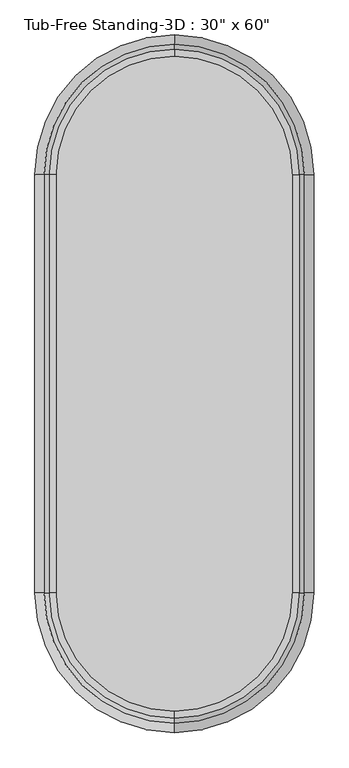
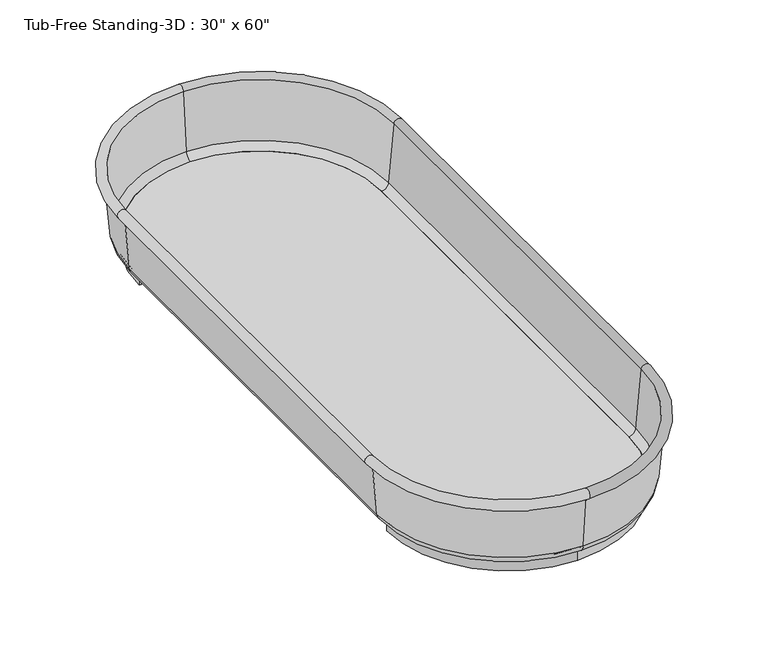
"""IFC4 building model written with IfcOpenShell, lengths in millimetres: flow terminal geometry."""

from ifc_helpers import new_model, si_unit, point, frame, frame_2d, origin, origin_with_axes, place, context, project, spatial, polyline, circle_curve, ellipse_curve, trimmed, segment, composite_curve, outline, extrude, source, transform, mapped, element, save
from ifc_brep_helpers import plane_surface, cylinder_surface, revolved_surface, advanced_brep


def flow_terminal_2cf38851(model_context):
    return source(origin(), model_context, "Body", "SolidModel", [
        advanced_brep(
        [(0.0, -1866.9, 406.4), (723.9, -1143.0, 406.4), (736.6, -1143.0, 406.4), (0.0, -1879.6, 406.4), (0.0, -1841.1045038, 111.5561295), (698.1045038, -1143.0, 111.5561295), (0.0, -1788.2824236, 63.1536107), (645.2824236, -1143.0, 63.1536107), (0.0, -1788.2824236, 78.0774627), (645.2824236, -1143.0, 78.0774627), (0.0, -1826.2374416, 112.8568289), (683.2374416, -1143.0, 112.8568289), (0.0, -1854.4561556, 435.3982063), (711.4561556, -1143.0, 435.3982063), (-723.9, -1143.0, 406.4), (-736.6, -1143.0, 406.4), (-698.1045038, -1143.0, 111.5561295), (-645.2824236, -1143.0, 63.1536107), (-645.2824236, -1143.0, 78.0774627), (-683.2374416, -1143.0, 112.8568289), (-711.4561556, -1143.0, 435.3982063), (-736.6, 1143.0, 406.4), (-723.9, 1143.0, 406.4), (-698.1045038, 1143.0, 111.5561295), (-645.2824236, 1143.0, 63.1536107), (-645.2824236, 1143.0, 78.0774627), (-683.2374416, 1143.0, 112.8568289), (-711.4561556, 1143.0, 435.3982063), (0.0, 1866.9, 406.4), (0.0, 1879.6, 406.4), (0.0, 1841.1045038, 111.5561295), (0.0, 1788.2824236, 63.1536107), (0.0, 1788.2824236, 78.0774627), (0.0, 1826.2374416, 112.8568289), (0.0, 1854.4561556, 435.3982063), (723.9, 1143.0, 406.4), (736.6, 1143.0, 406.4), (698.1045038, 1143.0, 111.5561295), (645.2824236, 1143.0, 63.1536107), (645.2824236, 1143.0, 78.0774627), (683.2374416, 1143.0, 112.8568289), (711.4561556, 1143.0, 435.3982063)],
        [
            (0, 1, circle_curve(frame((0.0, -1143.0, 406.4), z_axis=(0.0, 0.0, 1.0), x_axis=(1.0, 0.0, 0.0)), 723.9)),
            (1, 2),
            (2, 3, circle_curve(frame((0.0, -1143.0, 406.4), z_axis=(0.0, 0.0, -1.0), x_axis=(1.0, 0.0, 0.0)), 736.6)),
            (3, 0),
            (4, 5, circle_curve(frame((0.0, -1143.0, 111.5561295), z_axis=(0.0, 0.0, 1.0), x_axis=(1.0, 0.0, 0.0)), 698.1045038)),
            (5, 1),
            (0, 4),
            (6, 7, circle_curve(frame((0.0, -1143.0, 63.1536107), z_axis=(0.0, 0.0, 1.0), x_axis=(1.0, 0.0, 0.0)), 645.2824236)),
            (7, 5, circle_curve(frame((645.2824236, -1143.0, 116.1774627), z_axis=(0.0, -1.0, 0.0), x_axis=(1.0, 0.0, 0.0)), 53.023852)),
            (4, 6, circle_curve(frame((0.0, -1788.2824236, 116.1774627), z_axis=(1.0, 0.0, 0.0), x_axis=(0.0, -1.0, 0.0)), 53.023852)),
            (8, 9, circle_curve(frame((0.0, -1143.0, 78.0774627), z_axis=(0.0, 0.0, 1.0), x_axis=(1.0, 0.0, 0.0)), 645.2824236)),
            (9, 7),
            (6, 8),
            (10, 11, circle_curve(frame((0.0, -1143.0, 112.8568289), z_axis=(0.0, 0.0, 1.0), x_axis=(1.0, 0.0, 0.0)), 683.2374416)),
            (11, 9, circle_curve(frame((645.2824236, -1143.0, 116.1774627), z_axis=(0.0, 1.0, 0.0), x_axis=(1.0, 0.0, 0.0)), 38.1)),
            (8, 10, circle_curve(frame((0.0, -1788.2824236, 116.1774627), z_axis=(-1.0, 0.0, 0.0), x_axis=(0.0, -1.0, 0.0)), 38.1)),
            (12, 13, circle_curve(frame((0.0, -1143.0, 435.3982063), z_axis=(0.0, 0.0, 1.0), x_axis=(1.0, 0.0, 0.0)), 711.4561556)),
            (13, 11),
            (10, 12),
            (2, 13, circle_curve(frame((736.6, -1143.0, 431.8), z_axis=(0.0, -1.0, 0.0), x_axis=(1.0, 0.0, 0.0)), 25.4)),
            (12, 3, circle_curve(frame((0.0, -1879.6, 431.8), z_axis=(1.0, 0.0, 0.0), x_axis=(0.0, -1.0, 0.0)), 25.4)),
            (14, 0, circle_curve(frame((0.0, -1143.0, 406.4), z_axis=(0.0, 0.0, 1.0), x_axis=(0.0, -1.0, 0.0)), 723.9)),
            (3, 15, circle_curve(frame((0.0, -1143.0, 406.4), z_axis=(0.0, 0.0, -1.0), x_axis=(0.0, -1.0, 0.0)), 736.6)),
            (15, 14),
            (16, 4, circle_curve(frame((0.0, -1143.0, 111.5561295), z_axis=(0.0, 0.0, 1.0), x_axis=(0.0, -1.0, 0.0)), 698.1045038)),
            (14, 16),
            (17, 6, circle_curve(frame((0.0, -1143.0, 63.1536107), z_axis=(0.0, 0.0, 1.0), x_axis=(0.0, -1.0, 0.0)), 645.2824236)),
            (16, 17, circle_curve(frame((-645.2824236, -1143.0, 116.1774627), z_axis=(0.0, -1.0, 0.0), x_axis=(-1.0, 0.0, 0.0)), 53.023852)),
            (18, 8, circle_curve(frame((0.0, -1143.0, 78.0774627), z_axis=(0.0, 0.0, 1.0), x_axis=(0.0, -1.0, 0.0)), 645.2824236)),
            (17, 18),
            (19, 10, circle_curve(frame((0.0, -1143.0, 112.8568289), z_axis=(0.0, 0.0, 1.0), x_axis=(0.0, -1.0, 0.0)), 683.2374416)),
            (18, 19, circle_curve(frame((-645.2824236, -1143.0, 116.1774627), z_axis=(0.0, 1.0, 0.0), x_axis=(-1.0, 0.0, 0.0)), 38.1)),
            (20, 12, circle_curve(frame((0.0, -1143.0, 435.3982063), z_axis=(0.0, 0.0, 1.0), x_axis=(0.0, -1.0, 0.0)), 711.4561556)),
            (19, 20),
            (20, 15, circle_curve(frame((-736.6, -1143.0, 431.8), z_axis=(0.0, -1.0, 0.0), x_axis=(-1.0, 0.0, 0.0)), 25.4)),
            (15, 21),
            (21, 22),
            (22, 14),
            (22, 23),
            (23, 16),
            (23, 24, circle_curve(frame((-645.2824236, 1143.0, 116.1774627), z_axis=(0.0, -1.0, 0.0), x_axis=(-1.0, 0.0, 0.0)), 53.023852)),
            (24, 17),
            (24, 25),
            (25, 18),
            (25, 26, circle_curve(frame((-645.2824236, 1143.0, 116.1774627), z_axis=(0.0, 1.0, 0.0), x_axis=(-1.0, 0.0, 0.0)), 38.1)),
            (26, 19),
            (26, 27),
            (27, 20),
            (27, 21, circle_curve(frame((-736.6, 1143.0, 431.8), z_axis=(0.0, -1.0, 0.0), x_axis=(-1.0, 0.0, 0.0)), 25.4)),
            (28, 22, circle_curve(frame((0.0, 1143.0, 406.4), z_axis=(0.0, 0.0, 1.0), x_axis=(-1.0, 0.0, 0.0)), 723.9)),
            (21, 29, circle_curve(frame((0.0, 1143.0, 406.4), z_axis=(0.0, 0.0, -1.0), x_axis=(-1.0, 0.0, 0.0)), 736.6)),
            (29, 28),
            (30, 23, circle_curve(frame((0.0, 1143.0, 111.5561295), z_axis=(0.0, 0.0, 1.0), x_axis=(-1.0, 0.0, 0.0)), 698.1045038)),
            (28, 30),
            (31, 24, circle_curve(frame((0.0, 1143.0, 63.1536107), z_axis=(0.0, 0.0, 1.0), x_axis=(-1.0, 0.0, 0.0)), 645.2824236)),
            (30, 31, circle_curve(frame((0.0, 1788.2824236, 116.1774627), z_axis=(-1.0, 0.0, 0.0), x_axis=(0.0, 1.0, 0.0)), 53.023852)),
            (32, 25, circle_curve(frame((0.0, 1143.0, 78.0774627), z_axis=(0.0, 0.0, 1.0), x_axis=(-1.0, 0.0, 0.0)), 645.2824236)),
            (31, 32),
            (33, 26, circle_curve(frame((0.0, 1143.0, 112.8568289), z_axis=(0.0, 0.0, 1.0), x_axis=(-1.0, 0.0, 0.0)), 683.2374416)),
            (32, 33, circle_curve(frame((0.0, 1788.2824236, 116.1774627), z_axis=(1.0, 0.0, 0.0), x_axis=(0.0, 1.0, 0.0)), 38.1)),
            (34, 27, circle_curve(frame((0.0, 1143.0, 435.3982063), z_axis=(0.0, 0.0, 1.0), x_axis=(-1.0, 0.0, 0.0)), 711.4561556)),
            (33, 34),
            (34, 29, circle_curve(frame((0.0, 1879.6, 431.8), z_axis=(-1.0, 0.0, 0.0), x_axis=(0.0, 1.0, 0.0)), 25.4)),
            (35, 28, circle_curve(frame((0.0, 1143.0, 406.4), z_axis=(0.0, 0.0, 1.0), x_axis=(0.0, 1.0, 0.0)), 723.9)),
            (29, 36, circle_curve(frame((0.0, 1143.0, 406.4), z_axis=(0.0, 0.0, -1.0), x_axis=(0.0, 1.0, 0.0)), 736.6)),
            (36, 35),
            (37, 30, circle_curve(frame((0.0, 1143.0, 111.5561295), z_axis=(0.0, 0.0, 1.0), x_axis=(0.0, 1.0, 0.0)), 698.1045038)),
            (35, 37),
            (38, 31, circle_curve(frame((0.0, 1143.0, 63.1536107), z_axis=(0.0, 0.0, 1.0), x_axis=(0.0, 1.0, 0.0)), 645.2824236)),
            (37, 38, circle_curve(frame((645.2824236, 1143.0, 116.1774627), z_axis=(0.0, 1.0, 0.0), x_axis=(1.0, 0.0, 0.0)), 53.023852)),
            (39, 32, circle_curve(frame((0.0, 1143.0, 78.0774627), z_axis=(0.0, 0.0, 1.0), x_axis=(0.0, 1.0, 0.0)), 645.2824236)),
            (38, 39),
            (40, 33, circle_curve(frame((0.0, 1143.0, 112.8568289), z_axis=(0.0, 0.0, 1.0), x_axis=(0.0, 1.0, 0.0)), 683.2374416)),
            (39, 40, circle_curve(frame((645.2824236, 1143.0, 116.1774627), z_axis=(0.0, -1.0, 0.0), x_axis=(1.0, 0.0, 0.0)), 38.1)),
            (41, 34, circle_curve(frame((0.0, 1143.0, 435.3982063), z_axis=(0.0, 0.0, 1.0), x_axis=(0.0, 1.0, 0.0)), 711.4561556)),
            (40, 41),
            (41, 36, circle_curve(frame((736.6, 1143.0, 431.8), z_axis=(0.0, 1.0, 0.0), x_axis=(1.0, 0.0, 0.0)), 25.4)),
            (36, 2),
            (1, 35),
            (5, 37),
            (7, 38),
            (9, 39),
            (11, 40),
            (13, 41),
        ],
        [
            plane_surface(frame((0.0, -1143.0, 406.4), z_axis=(0.0, 0.0, -1.0), x_axis=(1.0, 0.0, 0.0))),
            revolved_surface(polyline([(723.9, -1143.0, 406.4), (698.1045038, -1143.0, 111.5561295)]), (0.0, -1143.0, 431.8), (0.0, 0.0, -1.0)),
            revolved_surface(trimmed(ellipse_curve(frame((645.2824236, -1143.0, 116.1774627), z_axis=(0.0, 1.0, 0.0), x_axis=(1.0, 0.0, 0.0)), 53.023852, 53.023852), [point((698.1045038, -1143.0, 111.5561295))], [point((645.2824236, -1143.0, 63.1536107))], True, "CARTESIAN"), (0.0, -1143.0, 431.8), (0.0, 0.0, -1.0)),
            revolved_surface(polyline([(645.2824236, -1143.0, 63.1536107), (645.2824236, -1143.0, 78.07746270000001)]), (0.0, -1143.0, 431.8), (0.0, 0.0, -1.0)),
            revolved_surface(trimmed(ellipse_curve(frame((645.2824236, -1143.0, 116.1774627), z_axis=(0.0, -1.0, 0.0), x_axis=(1.0, 0.0, 0.0)), 38.1, 38.1), [point((645.2824236, -1143.0, 78.0774627))], [point((683.2374416, -1143.0, 112.8568289))], True, "CARTESIAN"), (0.0, -1143.0, 431.8), (0.0, 0.0, -1.0)),
            revolved_surface(polyline([(683.2374416, -1143.0, 112.8568289), (711.4561556, -1143.0, 435.3982063)]), (0.0, -1143.0, 431.8), (0.0, 0.0, -1.0)),
            revolved_surface(trimmed(ellipse_curve(frame((736.6, -1143.0, 431.8), z_axis=(0.0, 1.0, 0.0), x_axis=(1.0, 0.0, 0.0)), 25.4, 25.4), [point((711.4561556, -1143.0, 435.3982063))], [point((736.6, -1143.0, 406.4))], True, "CARTESIAN"), (0.0, -1143.0, 431.8), (0.0, 0.0, -1.0)),
            plane_surface(frame((0.0, -1143.0, 406.4), z_axis=(0.0, 0.0, -1.0), x_axis=(0.0, -1.0, 0.0))),
            revolved_surface(polyline([(0.0, -1866.9, 406.4), (0.0, -1841.1045038, 111.5561295)]), (0.0, -1143.0, 431.8), (0.0, 0.0, -1.0)),
            revolved_surface(trimmed(ellipse_curve(frame((0.0, -1788.2824236, 116.1774627), z_axis=(1.0, 0.0, 0.0), x_axis=(0.0, -1.0, 0.0)), 53.023852, 53.023852), [point((0.0, -1841.1045038, 111.5561295))], [point((0.0, -1788.2824236, 63.1536107))], True, "CARTESIAN"), (0.0, -1143.0, 431.8), (0.0, 0.0, -1.0)),
            revolved_surface(polyline([(0.0, -1788.2824236000001, 63.1536107), (0.0, -1788.2824236000001, 78.07746270000001)]), (0.0, -1143.0, 431.8), (0.0, 0.0, -1.0)),
            revolved_surface(trimmed(ellipse_curve(frame((0.0, -1788.2824236, 116.1774627), z_axis=(-1.0, 0.0, 0.0), x_axis=(0.0, -1.0, 0.0)), 38.1, 38.1), [point((0.0, -1788.2824236, 78.0774627))], [point((0.0, -1826.2374416, 112.8568289))], True, "CARTESIAN"), (0.0, -1143.0, 431.8), (0.0, 0.0, -1.0)),
            revolved_surface(polyline([(0.0, -1826.2374416, 112.8568289), (0.0, -1854.4561556, 435.3982063)]), (0.0, -1143.0, 431.8), (0.0, 0.0, -1.0)),
            revolved_surface(trimmed(ellipse_curve(frame((0.0, -1879.6, 431.8), z_axis=(1.0, 0.0, 0.0), x_axis=(0.0, -1.0, 0.0)), 25.4, 25.4), [point((0.0, -1854.4561556, 435.3982063))], [point((0.0, -1879.6, 406.4))], True, "CARTESIAN"), (0.0, -1143.0, 431.8), (0.0, 0.0, -1.0)),
            plane_surface(frame((-736.6, -1143.0, 406.4), z_axis=(0.0, 0.0, -1.0), x_axis=(0.0, 1.0, 0.0))),
            plane_surface(frame((-723.9, -1143.0, 406.4), z_axis=(-0.9961946980917455, 0.0, -0.08715574274765882), x_axis=(0.0, 1.0, 0.0))),
            cylinder_surface(frame((-645.2824236, -1143.0, 116.1774627), z_axis=(0.0, -1.0, 0.0), x_axis=(-1.0, 0.0, 0.0)), 53.023852),
            plane_surface(frame((-645.2824236, -1143.0, 63.1536107), z_axis=(1.0, 0.0, 0.0), x_axis=(0.0, 1.0, 0.0))),
            revolved_surface(polyline([(-683.3824236, 1143.0, 116.1774627), (-683.3824236, -1143.0, 116.1774627)]), (-645.2824236, -1143.0, 116.1774627), (0.0, 1.0, 0.0)),
            plane_surface(frame((-683.2374416, -1143.0, 112.8568289), z_axis=(0.9961946980917457, 0.0, 0.08715574274765676), x_axis=(0.0, 1.0, 0.0))),
            cylinder_surface(frame((-736.6, -1143.0, 431.8), z_axis=(0.0, -1.0, 0.0), x_axis=(-1.0, 0.0, 0.0)), 25.4),
            plane_surface(frame((0.0, 1143.0, 406.4), z_axis=(0.0, 0.0, -1.0), x_axis=(-1.0, 0.0, 0.0))),
            revolved_surface(polyline([(-723.9, 1143.0, 406.4), (-698.1045038, 1143.0, 111.5561295)]), (0.0, 1143.0, 431.8), (0.0, 0.0, -1.0)),
            revolved_surface(trimmed(ellipse_curve(frame((-645.2824236, 1143.0, 116.1774627), z_axis=(0.0, -1.0, 0.0), x_axis=(-1.0, 0.0, 0.0)), 53.023852, 53.023852), [point((-698.1045038, 1143.0, 111.5561295))], [point((-645.2824236, 1143.0, 63.1536107))], True, "CARTESIAN"), (0.0, 1143.0, 431.8), (0.0, 0.0, -1.0)),
            revolved_surface(polyline([(-645.2824236, 1143.0, 63.1536107), (-645.2824236, 1143.0, 78.07746270000001)]), (0.0, 1143.0, 431.8), (0.0, 0.0, -1.0)),
            revolved_surface(trimmed(ellipse_curve(frame((-645.2824236, 1143.0, 116.1774627), z_axis=(0.0, 1.0, 0.0), x_axis=(-1.0, 0.0, 0.0)), 38.1, 38.1), [point((-645.2824236, 1143.0, 78.0774627))], [point((-683.2374416, 1143.0, 112.8568289))], True, "CARTESIAN"), (0.0, 1143.0, 431.8), (0.0, 0.0, -1.0)),
            revolved_surface(polyline([(-683.2374416, 1143.0, 112.8568289), (-711.4561556, 1143.0, 435.3982063)]), (0.0, 1143.0, 431.8), (0.0, 0.0, -1.0)),
            revolved_surface(trimmed(ellipse_curve(frame((-736.6, 1143.0, 431.8), z_axis=(0.0, -1.0, 0.0), x_axis=(-1.0, 0.0, 0.0)), 25.4, 25.4), [point((-711.4561556, 1143.0, 435.3982063))], [point((-736.6, 1143.0, 406.4))], True, "CARTESIAN"), (0.0, 1143.0, 431.8), (0.0, 0.0, -1.0)),
            plane_surface(frame((0.0, 1143.0, 406.4), z_axis=(0.0, 0.0, -1.0), x_axis=(0.0, 1.0, 0.0))),
            revolved_surface(polyline([(0.0, 1866.9, 406.4), (0.0, 1841.1045038, 111.5561295)]), (0.0, 1143.0, 431.8), (0.0, 0.0, -1.0)),
            revolved_surface(trimmed(ellipse_curve(frame((0.0, 1788.2824236, 116.1774627), z_axis=(-1.0, 0.0, 0.0), x_axis=(0.0, 1.0, 0.0)), 53.023852, 53.023852), [point((0.0, 1841.1045038, 111.5561295))], [point((0.0, 1788.2824236, 63.1536107))], True, "CARTESIAN"), (0.0, 1143.0, 431.8), (0.0, 0.0, -1.0)),
            revolved_surface(polyline([(0.0, 1788.2824236000001, 63.1536107), (0.0, 1788.2824236000001, 78.07746270000001)]), (0.0, 1143.0, 431.8), (0.0, 0.0, -1.0)),
            revolved_surface(trimmed(ellipse_curve(frame((0.0, 1788.2824236, 116.1774627), z_axis=(1.0, 0.0, 0.0), x_axis=(0.0, 1.0, 0.0)), 38.1, 38.1), [point((0.0, 1788.2824236, 78.0774627))], [point((0.0, 1826.2374416, 112.8568289))], True, "CARTESIAN"), (0.0, 1143.0, 431.8), (0.0, 0.0, -1.0)),
            revolved_surface(polyline([(0.0, 1826.2374416, 112.8568289), (0.0, 1854.4561556, 435.3982063)]), (0.0, 1143.0, 431.8), (0.0, 0.0, -1.0)),
            revolved_surface(trimmed(ellipse_curve(frame((0.0, 1879.6, 431.8), z_axis=(-1.0, 0.0, 0.0), x_axis=(0.0, 1.0, 0.0)), 25.4, 25.4), [point((0.0, 1854.4561556, 435.3982063))], [point((0.0, 1879.6, 406.4))], True, "CARTESIAN"), (0.0, 1143.0, 431.8), (0.0, 0.0, -1.0)),
            plane_surface(frame((736.6, 1143.0, 406.4), z_axis=(0.0, 0.0, -1.0), x_axis=(0.0, -1.0, 0.0))),
            plane_surface(frame((723.9, 1143.0, 406.4), z_axis=(0.9961946980917455, 0.0, -0.08715574274765882), x_axis=(0.0, -1.0, 0.0))),
            cylinder_surface(frame((645.2824236, 1143.0, 116.1774627), z_axis=(0.0, 1.0, 0.0), x_axis=(1.0, 0.0, 0.0)), 53.023852),
            plane_surface(frame((645.2824236, 1143.0, 63.1536107), z_axis=(-1.0, 0.0, 0.0), x_axis=(0.0, -1.0, 0.0))),
            revolved_surface(polyline([(683.3824236, -1143.0, 116.1774627), (683.3824236, 1143.0, 116.1774627)]), (645.2824236, 1143.0, 116.1774627), (0.0, -1.0, 0.0)),
            plane_surface(frame((683.2374416, 1143.0, 112.8568289), z_axis=(-0.9961946980917458, 0.0, 0.08715574274765678), x_axis=(0.0, -1.0, 0.0))),
            cylinder_surface(frame((736.6, 1143.0, 431.8), z_axis=(0.0, 1.0, 0.0), x_axis=(1.0, 0.0, 0.0)), 25.4),
        ],
        [
            (0, [[1, 2, 3, 4]]),
            (1, [[5, 6, -1, 7]]),
            (2, [[8, 9, -5, 10]]),
            (3, [[11, 12, -8, 13]]),
            (4, [[14, 15, -11, 16]]),
            (5, [[17, 18, -14, 19]]),
            (6, [[-3, 20, -17, 21]]),
            (7, [[22, -4, 23, 24]]),
            (8, [[25, -7, -22, 26]]),
            (9, [[27, -10, -25, 28]]),
            (10, [[29, -13, -27, 30]]),
            (11, [[31, -16, -29, 32]]),
            (12, [[33, -19, -31, 34]]),
            (13, [[-23, -21, -33, 35]]),
            (14, [[-24, 36, 37, 38]]),
            (15, [[-26, -38, 39, 40]]),
            (16, [[-28, -40, 41, 42]]),
            (17, [[-30, -42, 43, 44]]),
            (18, [[-32, -44, 45, 46]]),
            (19, [[-34, -46, 47, 48]]),
            (20, [[-35, -48, 49, -36]]),
            (21, [[50, -37, 51, 52]]),
            (22, [[53, -39, -50, 54]]),
            (23, [[55, -41, -53, 56]]),
            (24, [[57, -43, -55, 58]]),
            (25, [[59, -45, -57, 60]]),
            (26, [[61, -47, -59, 62]]),
            (27, [[-51, -49, -61, 63]]),
            (28, [[64, -52, 65, 66]]),
            (29, [[67, -54, -64, 68]]),
            (30, [[69, -56, -67, 70]]),
            (31, [[71, -58, -69, 72]]),
            (32, [[73, -60, -71, 74]]),
            (33, [[75, -62, -73, 76]]),
            (34, [[-65, -63, -75, 77]]),
            (35, [[-66, 78, -2, 79]]),
            (36, [[-68, -79, -6, 80]]),
            (37, [[-70, -80, -9, 81]]),
            (38, [[-72, -81, -12, 82]]),
            (39, [[-74, -82, -15, 83]]),
            (40, [[-76, -83, -18, 84]]),
            (41, [[-77, -84, -20, -78]]),
        ],
    ),
        extrude(outline(composite_curve([segment(polyline([(-645.2824236, -1143.0), (-645.2824236, 1143.0)]), True, "CONTINUOUS"), segment(trimmed(circle_curve(frame_2d((0.0, 1143.0)), 645.2824236), [point((-645.2824236, 1143.0))], [point((0.0, 1788.2824236))], False, "CARTESIAN"), True, "CONTINUOUS"), segment(trimmed(circle_curve(frame_2d((0.0, 1143.0)), 645.2824236), [point((0.0, 1788.2824236))], [point((645.2824236, 1143.0))], False, "CARTESIAN"), True, "CONTINUOUS"), segment(polyline([(645.2824236, 1143.0), (645.2824236, -1143.0)]), True, "CONTINUOUS"), segment(trimmed(circle_curve(frame_2d((0.0, -1143.0)), 645.2824236), [point((645.2824236, -1143.0))], [point((0.0, -1788.2824236))], False, "CARTESIAN"), True, "CONTINUOUS"), segment(trimmed(circle_curve(frame_2d((0.0, -1143.0)), 645.2824236), [point((0.0, -1788.2824236))], [point((-645.2824236, -1143.0))], False, "CARTESIAN"), True, "CONTINUOUS")], self_intersect=False)), frame((0.0, 0.0, 63.5), z_axis=(0.0, 0.0, 1.0), x_axis=(1.0, 0.0, 0.0)), (0.0, 0.0, 1.0), 15.08125),
        extrude(outline(composite_curve([segment(trimmed(circle_curve(frame_2d((0.0, -1143.0)), 645.2824236), [point((0.0, -1788.2824236))], [point((-645.2824236, -1143.0))], False, "CARTESIAN"), True, "CONTINUOUS"), segment(polyline([(-645.2824236, -1143.0), (-635.0, -1143.0)]), True, "CONTINUOUS"), segment(trimmed(circle_curve(frame_2d((0.0, -1143.0)), 635.0), [point((-635.0, -1143.0))], [point((0.0, -1778.0))], True, "CARTESIAN"), True, "CONTINUOUS"), segment(trimmed(circle_curve(frame_2d((0.0, -1143.0)), 635.0), [point((0.0, -1778.0))], [point((635.0, -1143.0))], True, "CARTESIAN"), True, "CONTINUOUS"), segment(polyline([(635.0, -1143.0), (645.2824236, -1143.0)]), True, "CONTINUOUS"), segment(trimmed(circle_curve(frame_2d((0.0, -1143.0)), 645.2824236), [point((645.2824236, -1143.0))], [point((0.0, -1788.2824236))], False, "CARTESIAN"), True, "CONTINUOUS")], self_intersect=False)), origin_with_axes(), (0.0, 0.0, 1.0), 63.5),
        extrude(outline(composite_curve([segment(trimmed(circle_curve(frame_2d((0.0, 1143.0)), 635.0), [point((0.0, 1778.0))], [point((-635.0, 1143.0))], True, "CARTESIAN"), True, "CONTINUOUS"), segment(polyline([(-635.0, 1143.0), (-645.2824236, 1143.0)]), True, "CONTINUOUS"), segment(trimmed(circle_curve(frame_2d((0.0, 1143.0)), 645.2824236), [point((-645.2824236, 1143.0))], [point((0.0, 1788.2824236))], False, "CARTESIAN"), True, "CONTINUOUS"), segment(trimmed(circle_curve(frame_2d((0.0, 1143.0)), 645.2824236), [point((0.0, 1788.2824236))], [point((645.2824236, 1143.0))], False, "CARTESIAN"), True, "CONTINUOUS"), segment(polyline([(645.2824236, 1143.0), (635.0, 1143.0)]), True, "CONTINUOUS"), segment(trimmed(circle_curve(frame_2d((0.0, 1143.0)), 635.0), [point((635.0, 1143.0))], [point((0.0, 1778.0))], True, "CARTESIAN"), True, "CONTINUOUS")], self_intersect=False)), origin_with_axes(), (0.0, 0.0, 1.0), 63.5),
    ])


if __name__ == "__main__":
    model = new_model("IFC4")
    model_context = context("Model", 3, world=origin())
    ifc_project = project(units=[si_unit("LENGTHUNIT", "METRE", prefix="MILLI")], contexts=[model_context])
    site = spatial("IfcSite", under=ifc_project)
    building = spatial("IfcBuilding", under=site)
    placement = place(None, origin())
    flow_terminal_shape = flow_terminal_2cf38851(model_context)
    element("IfcFlowTerminal", 1, ObjectType="Tub-Free Standing-3D : 30\" x 60\"", at=placement, inside=building, context=model_context, shape_type="MappedRepresentation", body=[
        mapped(flow_terminal_shape, transform((0.0, 0.0, 0.0), x_axis=(1.0, 0.0, 0.0), y_axis=(0.0, 1.0, 0.0), z_axis=(0.0, 0.0, 1.0))),
    ])
    save(model, "model.ifc")

# Revit data of these elements
# Type "Tub-Free Standing-3D : 30\" x 60\""
#   Assembly Code = "D2010110"
#   Height = 1' - 6"
#   Length = 12' - 6"
#   Width = 5' - 0"
#   Tub Material = Porcelain, Ivory
#   Default Elevation = 0
# Element 1 (IfcFlowTerminal, "Tub-Free Standing-3D : 30\" x 60\"")
#   Materials on its faces: "Porcelain, Ivory"
# Materials
#   "Porcelain, Ivory": class "Ceramic", colour RGB 247 247 239, transparency 0, Description = "Porcelain, ivory", Cost = 0
